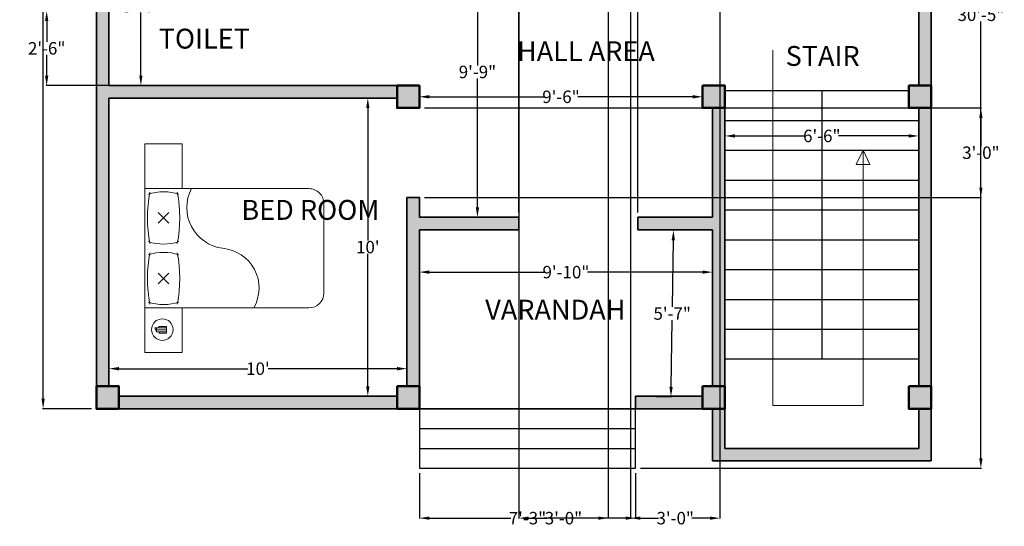
# Model space of a CAD drawing. Units: inches. Extents: x 157 to 553, y 100 to 520.
# Tile 1 of 2: x 157 to 553, y 100 to 304. Entities that reach past the tile are written whole.
import ezdxf

# ---------------------------------------------------------------- set-up
doc = ezdxf.new("R2010")
doc.units = ezdxf.units.IN
doc.header["$MEASUREMENT"] = 0
doc.layers.get('0').update_dxf_attribs({"color": 255})
for name, color, linetype, lineweight in [('A-ANNO-DIMS', 2, 'Continuous', 18), ('A-ANNO-SYMB', 2, 'Continuous', 18), ('A-AREA-IDEN', 7, 'Continuous', 25), ('A-COLS', 7, 'Continuous', 50), ('A-FLOR-STRS', 7, 'Continuous', 25), ('A-FURN', 3, 'Continuous', 18), ('A-WALL', 7, 'Continuous', 35), ('A-WALL-PATT', 3, 'Continuous', 13)]:
    doc.layers.add(name, color=color, linetype=linetype, lineweight=lineweight)
doc.layers.add('A-COLS-PATT', color=18, linetype='Continuous', lineweight=13, true_color=0x000000)
doc.styles.get("Standard").update_dxf_attribs({"font": 'arial.ttf'})
doc.dimstyles.get("Standard").update_dxf_attribs({"dimtxt": 5, "dimasz": 4, "dimexe": 0.18, "dimexo": 2, "dimgap": 0.09, "dimtad": 0, "dimtih": 1, "dimtoh": 1, "dimdec": 0, "dimzin": 0, "dimdsep": 46, "dimlunit": 3, "dimtxsty": 'Standard', "dimcen": 2, "dimadec": 0, "dimazin": 0, "dimtfac": 1, "dimtdec": 0, "dimtofl": 0, "dimtmove": 0, "dimatfit": 3, "dimfxl": 1, "dimtolj": 1, "dimtzin": 0, "dimarcsym": 0})

# ---------------------------------------------------------------- blocks, each defined once
blk = doc.blocks.new('*D2')
at = {"layer": 'A-ANNO-DIMS', "color": 0, "lineweight": -2, "transparency": 16777216}
for p, q in [((185.79, 488.7), (166.12, 488.7)), ((166.3, 484.7), (166.3, 320.85)), ((166.3, 151.7), (166.3, 315.56)), ((185.79, 147.7), (166.12, 147.7))]:
    blk.add_line(p, q, dxfattribs=at)
at = {"layer": 'A-ANNO-DIMS', "color": 0, "transparency": 16777216}
for points in [[(165.64, 484.7), (166.97, 484.7), (166.3, 488.7)], [(165.64, 151.7), (166.97, 151.7), (166.3, 147.7)]]:
    blk.add_solid(points, dxfattribs=at)
at = {"layer": 'Defpoints', "color": 0, "transparency": 16777216}
for p in [(187.79, 488.7), (166.3, 147.7), (187.79, 147.7)]:
    blk.add_point(p, dxfattribs=at)
at = {"layer": 'A-ANNO-DIMS', "color": 0, "transparency": 16777216, "insert": (166.3, 318.2), "char_height": 5, "attachment_point": 5}
blk.add_mtext('\\A1;28\'-5"', dxfattribs=at)
blk = doc.blocks.new('*D3')
at = {"layer": 'A-ANNO-DIMS', "color": 0, "lineweight": -2, "transparency": 16777216}
for p, q in [((440.79, 266.7), (440.79, 257.27)), ((518.79, 266.7), (518.79, 257.27)), ((444.79, 257.45), (473.04, 257.45)), ((514.79, 257.45), (486.54, 257.45))]:
    blk.add_line(p, q, dxfattribs=at)
at = {"layer": 'A-ANNO-DIMS', "color": 0, "transparency": 16777216}
for points in [[(444.79, 258.12), (444.79, 256.78), (440.79, 257.45)], [(514.79, 258.12), (514.79, 256.78), (518.79, 257.45)]]:
    blk.add_solid(points, dxfattribs=at)
at = {"layer": 'Defpoints', "color": 0, "transparency": 16777216}
for p in [(440.79, 268.7), (518.79, 268.7), (518.79, 257.45)]:
    blk.add_point(p, dxfattribs=at)
at = {"layer": 'A-ANNO-DIMS', "color": 0, "transparency": 16777216, "insert": (479.79, 257.45), "char_height": 5, "attachment_point": 5}
blk.add_mtext('\\A1;6\'-6"', dxfattribs=at)
blk = doc.blocks.new('*D13')
at = {"layer": 'A-ANNO-DIMS', "color": 0, "lineweight": -2, "transparency": 16777216}
for p, q in [((198.79, 341.7), (205.83, 341.7)), ((205.65, 337.7), (205.65, 312.34)), ((205.65, 281.7), (205.65, 307.07)), ((198.79, 277.7), (205.83, 277.7))]:
    blk.add_line(p, q, dxfattribs=at)
at = {"layer": 'A-ANNO-DIMS', "color": 0, "transparency": 16777216}
for points in [[(204.99, 337.7), (206.32, 337.7), (205.65, 341.7)], [(204.99, 281.7), (206.32, 281.7), (205.65, 277.7)]]:
    blk.add_solid(points, dxfattribs=at)
at = {"layer": 'Defpoints', "color": 0, "transparency": 16777216}
for p in [(196.79, 341.7), (196.79, 277.7), (205.65, 277.7)]:
    blk.add_point(p, dxfattribs=at)
at = {"layer": 'A-ANNO-DIMS', "color": 0, "transparency": 16777216, "insert": (205.65, 309.7), "char_height": 5, "attachment_point": 5}
blk.add_mtext('\\A1;5\'-4"', dxfattribs=at)
blk = doc.blocks.new('*D14')
at = {"layer": 'A-ANNO-DIMS', "color": 0, "lineweight": -2, "transparency": 16777216}
for p, q in [((192.79, 158.7), (192.79, 163.98)), ((196.79, 163.8), (248.69, 163.8)), ((308.79, 163.8), (256.89, 163.8)), ((312.79, 158.7), (312.79, 163.98))]:
    blk.add_line(p, q, dxfattribs=at)
at = {"layer": 'A-ANNO-DIMS', "color": 0, "transparency": 16777216}
for points in [[(196.79, 164.47), (196.79, 163.13), (192.79, 163.8)], [(308.79, 164.47), (308.79, 163.13), (312.79, 163.8)]]:
    blk.add_solid(points, dxfattribs=at)
at = {"layer": 'Defpoints', "color": 0, "transparency": 16777216}
for p in [(312.79, 163.8), (192.79, 156.7), (312.79, 156.7)]:
    blk.add_point(p, dxfattribs=at)
at = {"layer": 'A-ANNO-DIMS', "color": 0, "transparency": 16777216, "insert": (252.79, 163.8), "char_height": 5, "attachment_point": 5}
blk.add_mtext("\\A1;10'", dxfattribs=at)
blk = doc.blocks.new('*D15')
at = {"layer": 'A-ANNO-DIMS', "color": 0, "lineweight": -2, "transparency": 16777216}
for p, q in [((306.79, 272.7), (296.84, 272.7)), ((297.02, 268.7), (297.02, 215.35)), ((297.02, 156.7), (297.02, 210.06)), ((306.79, 152.7), (296.84, 152.7))]:
    blk.add_line(p, q, dxfattribs=at)
at = {"layer": 'A-ANNO-DIMS', "color": 0, "transparency": 16777216}
for points in [[(296.36, 268.7), (297.69, 268.7), (297.02, 272.7)], [(296.36, 156.7), (297.69, 156.7), (297.02, 152.7)]]:
    blk.add_solid(points, dxfattribs=at)
at = {"layer": 'Defpoints', "color": 0, "transparency": 16777216}
for p in [(297.02, 272.7), (308.79, 272.7), (308.79, 152.7)]:
    blk.add_point(p, dxfattribs=at)
at = {"layer": 'A-ANNO-DIMS', "color": 0, "transparency": 16777216, "insert": (297.02, 212.7), "char_height": 5, "attachment_point": 5}
blk.add_mtext("\\A1;10'", dxfattribs=at)
blk = doc.blocks.new('*D16')
at = {"layer": 'A-ANNO-DIMS', "color": 0, "lineweight": -2, "transparency": 16777216}
for p, q in [((317.79, 217.7), (317.79, 202.47)), ((435.79, 217.7), (435.79, 202.47)), ((321.79, 202.65), (368.11, 202.65)), ((431.79, 202.65), (385.47, 202.65))]:
    blk.add_line(p, q, dxfattribs=at)
at = {"layer": 'A-ANNO-DIMS', "color": 0, "transparency": 16777216}
for points in [[(321.79, 203.32), (321.79, 201.99), (317.79, 202.65)], [(431.79, 203.32), (431.79, 201.99), (435.79, 202.65)]]:
    blk.add_solid(points, dxfattribs=at)
at = {"layer": 'Defpoints', "color": 0, "transparency": 16777216}
for p in [(317.79, 219.7), (435.79, 219.7), (435.79, 202.65)]:
    blk.add_point(p, dxfattribs=at)
at = {"layer": 'A-ANNO-DIMS', "color": 0, "transparency": 16777216, "insert": (376.79, 202.65), "char_height": 5, "attachment_point": 5}
blk.add_mtext('\\A1;9\'-10"', dxfattribs=at)
blk = doc.blocks.new('*D17')
at = {"layer": 'A-ANNO-DIMS', "color": 0, "lineweight": -2, "transparency": 16777216}
for p, q in [((407.79, 219.67), (420.24, 219.49)), ((420, 215.49), (419.6, 188.62)), ((419.12, 156.49), (419.52, 183.36)), ((406.79, 152.67), (419.24, 152.49))]:
    blk.add_line(p, q, dxfattribs=at)
at = {"layer": 'A-ANNO-DIMS', "color": 0, "transparency": 16777216}
for points in [[(419.33, 215.5), (420.67, 215.48), (420.06, 219.49)], [(418.45, 156.5), (419.79, 156.48), (419.06, 152.49)]]:
    blk.add_solid(points, dxfattribs=at)
at = {"layer": 'Defpoints', "color": 0, "transparency": 16777216}
for p in [(405.79, 219.7), (420.06, 219.49), (404.79, 152.7)]:
    blk.add_point(p, dxfattribs=at)
at = {"layer": 'A-ANNO-DIMS', "color": 0, "transparency": 16777216, "insert": (419.56, 185.99), "char_height": 5, "attachment_point": 5}
blk.add_mtext('\\A1;5\'-7"', dxfattribs=at)
blk = doc.blocks.new('*D18')
at = {"layer": 'A-ANNO-DIMS', "color": 0, "lineweight": -2, "transparency": 16777216}
for p, q in [((355.79, 341.7), (340.98, 341.7)), ((341.16, 337.7), (341.16, 285.85)), ((341.16, 228.7), (341.16, 280.56)), ((355.79, 224.7), (340.98, 224.7))]:
    blk.add_line(p, q, dxfattribs=at)
at = {"layer": 'A-ANNO-DIMS', "color": 0, "transparency": 16777216}
for points in [[(340.49, 337.7), (341.82, 337.7), (341.16, 341.7)], [(340.49, 228.7), (341.82, 228.7), (341.16, 224.7)]]:
    blk.add_solid(points, dxfattribs=at)
at = {"layer": 'Defpoints', "color": 0, "transparency": 16777216}
for p in [(341.16, 341.7), (357.79, 341.7), (357.79, 224.7)]:
    blk.add_point(p, dxfattribs=at)
at = {"layer": 'A-ANNO-DIMS', "color": 0, "transparency": 16777216, "insert": (341.16, 283.2), "char_height": 5, "attachment_point": 5}
blk.add_mtext('\\A1;9\'-9"', dxfattribs=at)
blk = doc.blocks.new('*D19')
at = {"layer": 'A-ANNO-DIMS', "color": 0, "lineweight": -2, "transparency": 16777216}
for p, q in [((317.79, 270.7), (317.79, 273.38)), ((321.79, 273.2), (368.05, 273.2)), ((427.79, 273.2), (381.52, 273.2)), ((431.79, 270.7), (431.79, 273.38))]:
    blk.add_line(p, q, dxfattribs=at)
at = {"layer": 'A-ANNO-DIMS', "color": 0, "transparency": 16777216}
for points in [[(321.79, 273.87), (321.79, 272.54), (317.79, 273.2)], [(427.79, 273.87), (427.79, 272.54), (431.79, 273.2)]]:
    blk.add_solid(points, dxfattribs=at)
at = {"layer": 'Defpoints', "color": 0, "transparency": 16777216}
for p in [(431.79, 273.2), (317.79, 268.7), (431.79, 268.7)]:
    blk.add_point(p, dxfattribs=at)
at = {"layer": 'A-ANNO-DIMS', "color": 0, "transparency": 16777216, "insert": (374.79, 273.2), "char_height": 5, "attachment_point": 5}
blk.add_mtext('\\A1;9\'-6"', dxfattribs=at)
blk = doc.blocks.new('BED-DOUBLE-WITH-NIGHTSTANDS')
for p, q in [((0, 72), (18, 72)), ((0, 57), (0, 72)), ((6, 72), (84, 72)), ((18, 72), (18, 6)), ((66, 6), (66, 72)), ((84, 72), (84, 57)), ((9.95, 67.98), (8.32, 67.38)), ((9.95, 67.38), (9.95, 67.98)), ((9.14, 67.38), (9.14, 63.35)), ((32, 66.63), (27.75, 62.4)), ((27.76, 66.64), (31.99, 62.39)), ((56.35, 66.63), (52.1, 62.4)), ((52.11, 66.64), (56.34, 62.39)), ((18, 57), (0, 57)), ((84, 57), (66, 57)), ((24, 0), (60, 0))]:
    blk.add_line(p, q)
for points in [[(8.32, 63.35), (7.8, 63.35), (7.8, 66.31), (8.32, 66.31)], [(8.32, 63.35), (9.95, 63.35), (9.95, 67.38), (8.32, 67.38)], [(9.95, 63.35), (10.59, 63.35), (10.59, 66.42), (9.95, 66.42)]]:
    blk.add_lwpolyline(points, close=True)
blk.add_circle((9.27, 65.01), 4.35)
for centre, radius, start, end in [((54.23, 16.39), 56.63, 100.869, 100.8807), ((54.23, 16.39), 56.63, 79.1193, 79.131), ((40, 64.52), 20.63, 162.5077, 197.4923), ((29.88, 16.39), 54.63, 79.1193, 100.8807), ((19.75, 64.52), 20.62, 342.5077, 17.4923), ((64.35, 64.52), 20.63, 162.5077, 197.4923), ((54.23, 16.39), 54.63, 79.1193, 100.8807), ((44.1, 64.52), 20.62, 342.5077, 17.4923), ((29.88, 112.64), 54.63, 259.1193, 280.8807), ((54.23, 112.64), 54.63, 259.1193, 280.8807), ((58.39, 38.66), 16.52, 62.5747, 172.7011), ((25.97, 42.18), 16.1, 240.3431, 354.9328), ((24, 6), 6, 180, 270), ((60, 6), 6, 270, 0)]:
    blk.add_arc(centre, radius, start, end)
blk = doc.blocks.new('*D23')
at = {"layer": 'A-ANNO-DIMS', "color": 0, "lineweight": -2, "transparency": 16777216}
for p, q in [((525.79, 488.7), (544.02, 488.7)), ((543.84, 484.7), (543.84, 308.85)), ((543.84, 127.7), (543.84, 303.56)), ((406.79, 123.7), (544.02, 123.7))]:
    blk.add_line(p, q, dxfattribs=at)
at = {"layer": 'A-ANNO-DIMS', "color": 0, "transparency": 16777216}
for points in [[(543.17, 484.7), (544.5, 484.7), (543.84, 488.7)], [(543.17, 127.7), (544.5, 127.7), (543.84, 123.7)]]:
    blk.add_solid(points, dxfattribs=at)
at = {"layer": 'Defpoints', "color": 0, "transparency": 16777216}
for p in [(523.79, 488.7), (404.79, 123.7), (543.84, 123.7)]:
    blk.add_point(p, dxfattribs=at)
at = {"layer": 'A-ANNO-DIMS', "color": 0, "transparency": 16777216, "insert": (543.84, 306.2), "char_height": 5, "attachment_point": 5}
blk.add_mtext('\\A1;30\'-5"', dxfattribs=at)
blk = doc.blocks.new('*D25')
at = {"layer": 'A-ANNO-DIMS', "color": 0, "lineweight": -2, "transparency": 16777216}
for p, q in [((357.79, 339.7), (357.79, 103.47)), ((393.79, 339.7), (393.79, 103.47)), ((361.79, 103.65), (369.05, 103.65)), ((389.79, 103.65), (382.52, 103.65))]:
    blk.add_line(p, q, dxfattribs=at)
at = {"layer": 'A-ANNO-DIMS', "color": 0, "transparency": 16777216}
for points in [[(361.79, 104.32), (361.79, 102.99), (357.79, 103.65)], [(389.79, 104.32), (389.79, 102.99), (393.79, 103.65)]]:
    blk.add_solid(points, dxfattribs=at)
at = {"layer": 'Defpoints', "color": 0, "transparency": 16777216}
for p in [(357.79, 341.7), (393.79, 341.7), (393.79, 103.65)]:
    blk.add_point(p, dxfattribs=at)
at = {"layer": 'A-ANNO-DIMS', "color": 0, "transparency": 16777216, "insert": (375.79, 103.65), "char_height": 5, "attachment_point": 5}
blk.add_mtext('\\A1;3\'-0"', dxfattribs=at)
blk = doc.blocks.new('*D26')
at = {"layer": 'A-ANNO-DIMS', "color": 0, "lineweight": -2, "transparency": 16777216}
for p, q in [((402.79, 339.7), (402.79, 103.47)), ((438.79, 339.7), (438.79, 103.47)), ((406.79, 103.65), (414.05, 103.65)), ((434.79, 103.65), (427.52, 103.65))]:
    blk.add_line(p, q, dxfattribs=at)
at = {"layer": 'A-ANNO-DIMS', "color": 0, "transparency": 16777216}
for points in [[(406.79, 104.32), (406.79, 102.99), (402.79, 103.65)], [(434.79, 104.32), (434.79, 102.99), (438.79, 103.65)]]:
    blk.add_solid(points, dxfattribs=at)
at = {"layer": 'Defpoints', "color": 0, "transparency": 16777216}
for p in [(402.79, 341.7), (438.79, 341.7), (438.79, 103.65)]:
    blk.add_point(p, dxfattribs=at)
at = {"layer": 'A-ANNO-DIMS', "color": 0, "transparency": 16777216, "insert": (420.79, 103.65), "char_height": 5, "attachment_point": 5}
blk.add_mtext('\\A1;3\'-0"', dxfattribs=at)
blk = doc.blocks.new('*D27')
at = {"layer": 'A-ANNO-DIMS', "color": 0, "lineweight": -2, "transparency": 16777216}
for p, q in [((269.79, 307.7), (167.56, 307.7)), ((167.74, 303.7), (167.74, 295.35)), ((167.74, 281.7), (167.74, 290.06)), ((306.79, 277.7), (167.56, 277.7))]:
    blk.add_line(p, q, dxfattribs=at)
at = {"layer": 'A-ANNO-DIMS', "color": 0, "transparency": 16777216}
for points in [[(167.07, 303.7), (168.4, 303.7), (167.74, 307.7)], [(167.07, 281.7), (168.4, 281.7), (167.74, 277.7)]]:
    blk.add_solid(points, dxfattribs=at)
at = {"layer": 'Defpoints', "color": 0, "transparency": 16777216}
for p in [(271.79, 307.7), (167.74, 277.7), (308.79, 277.7)]:
    blk.add_point(p, dxfattribs=at)
at = {"layer": 'A-ANNO-DIMS', "color": 0, "transparency": 16777216, "insert": (167.74, 292.7), "char_height": 5, "attachment_point": 5}
blk.add_mtext('\\A1;2\'-6"', dxfattribs=at)
blk = doc.blocks.new('*D28')
at = {"layer": 'A-ANNO-DIMS', "color": 0, "lineweight": -2, "transparency": 16777216}
for p, q in [((319.79, 268.7), (544.02, 268.7)), ((543.84, 264.7), (543.84, 253.35)), ((543.84, 236.7), (543.84, 248.06)), ((319.79, 232.7), (544.02, 232.7))]:
    blk.add_line(p, q, dxfattribs=at)
at = {"layer": 'A-ANNO-DIMS', "color": 0, "transparency": 16777216}
for points in [[(543.17, 264.7), (544.5, 264.7), (543.84, 268.7)], [(543.17, 236.7), (544.5, 236.7), (543.84, 232.7)]]:
    blk.add_solid(points, dxfattribs=at)
at = {"layer": 'Defpoints', "color": 0, "transparency": 16777216}
for p in [(317.79, 268.7), (317.79, 232.7), (543.84, 232.7)]:
    blk.add_point(p, dxfattribs=at)
at = {"layer": 'A-ANNO-DIMS', "color": 0, "transparency": 16777216, "insert": (543.84, 250.7), "char_height": 5, "attachment_point": 5}
blk.add_mtext('\\A1;3\'-0"', dxfattribs=at)
blk = doc.blocks.new('*D29')
at = {"layer": 'A-ANNO-DIMS', "color": 0, "lineweight": -2, "transparency": 16777216}
for p, q in [((357.79, 226.7), (357.79, 508.93)), ((361.79, 508.75), (374.95, 508.75)), ((401.79, 508.75), (388.62, 508.75)), ((405.79, 226.7), (405.79, 508.93))]:
    blk.add_line(p, q, dxfattribs=at)
at = {"layer": 'A-ANNO-DIMS', "color": 0, "transparency": 16777216}
for points in [[(361.79, 509.42), (361.79, 508.09), (357.79, 508.75)], [(401.79, 509.42), (401.79, 508.09), (405.79, 508.75)]]:
    blk.add_solid(points, dxfattribs=at)
at = {"layer": 'Defpoints', "color": 0, "transparency": 16777216}
for p in [(405.79, 508.75), (357.79, 224.7), (405.79, 224.7)]:
    blk.add_point(p, dxfattribs=at)
at = {"layer": 'A-ANNO-DIMS', "color": 0, "transparency": 16777216, "insert": (381.79, 508.75), "char_height": 5, "attachment_point": 5}
blk.add_mtext('\\A1;4\'-0"', dxfattribs=at)
blk = doc.blocks.new('*D30')
at = {"layer": 'A-ANNO-DIMS', "color": 0, "lineweight": -2, "transparency": 16777216}
for p, q in [((317.79, 121.7), (317.79, 103.47)), ((404.79, 121.7), (404.79, 103.47)), ((321.79, 103.65), (354.57, 103.65)), ((400.79, 103.65), (368, 103.65))]:
    blk.add_line(p, q, dxfattribs=at)
at = {"layer": 'A-ANNO-DIMS', "color": 0, "transparency": 16777216}
for points in [[(321.79, 104.32), (321.79, 102.99), (317.79, 103.65)], [(400.79, 104.32), (400.79, 102.99), (404.79, 103.65)]]:
    blk.add_solid(points, dxfattribs=at)
at = {"layer": 'Defpoints', "color": 0, "transparency": 16777216}
for p in [(317.79, 123.7), (404.79, 123.7), (404.79, 103.65)]:
    blk.add_point(p, dxfattribs=at)
at = {"layer": 'A-ANNO-DIMS', "color": 0, "transparency": 16777216, "insert": (361.29, 103.65), "char_height": 5, "attachment_point": 5}
blk.add_mtext('\\A1;7\'-3"', dxfattribs=at)

msp = doc.modelspace()

# ---------------------------------------------------------------- hatches: boundary and pattern name
at = {"layer": 'A-COLS-PATT'}
h = msp.add_hatch(color=256, dxfattribs=at)
h.dxf.hatch_style = 1
h.paths.add_polyline_path([(196.79, 156.7), (187.79, 156.7), (187.79, 147.7), (196.79, 147.7)])
h.paths.add_polyline_path([(317.79, 156.7), (308.79, 156.7), (308.79, 147.7), (317.79, 147.7)])
h.paths.add_polyline_path([(440.79, 156.7), (431.79, 156.7), (431.79, 147.7), (440.79, 147.7)])
h.paths.add_polyline_path([(523.79, 156.7), (514.79, 156.7), (514.79, 147.7), (523.79, 147.7)])
h.paths.add_polyline_path([(523.79, 277.7), (514.79, 277.7), (514.79, 268.7), (523.79, 268.7)])
h.paths.add_polyline_path([(440.79, 277.7), (431.79, 277.7), (431.79, 268.7), (440.79, 268.7)])
h.paths.add_polyline_path([(317.79, 277.7), (308.79, 277.7), (308.79, 268.7), (317.79, 268.7)])
h.paths.add_polyline_path([(196.79, 350.7), (187.79, 350.7), (187.79, 341.7), (196.79, 341.7)])
h.paths.add_polyline_path([(317.79, 350.7), (308.79, 350.7), (308.79, 341.7), (317.79, 341.7)])
h.paths.add_polyline_path([(402.79, 350.7), (393.79, 350.7), (393.79, 341.7), (402.79, 341.7)])
h.paths.add_polyline_path([(523.79, 350.7), (514.79, 350.7), (514.79, 341.7), (523.79, 341.7)])
h.paths.add_polyline_path([(523.79, 488.7), (514.79, 488.7), (514.79, 479.7), (523.79, 479.7)])
h.paths.add_polyline_path([(402.79, 488.7), (393.79, 488.7), (393.79, 479.7), (402.79, 479.7)])
h.paths.add_polyline_path([(317.79, 488.7), (308.79, 488.7), (308.79, 479.7), (317.79, 479.7)])
h.paths.add_polyline_path([(196.79, 488.7), (187.79, 488.7), (187.79, 479.7), (196.79, 479.7)])
at = {"layer": 'A-WALL-PATT'}
h = msp.add_hatch(color=256, dxfattribs=at)
h.dxf.hatch_style = 1
h.paths.add_polyline_path([(271.79, 346.7), (196.79, 346.7), (196.79, 341.7), (266.79, 341.7), (266.79, 307.7), (271.79, 307.7)])
h.paths.add_polyline_path([(308.79, 277.7), (192.79, 277.7), (192.79, 341.7), (187.79, 341.7), (187.79, 156.7), (192.79, 156.7), (192.79, 272.7), (308.79, 272.7)])
h.paths.add_polyline_path([(357.79, 224.7), (317.79, 224.7), (317.79, 232.7), (312.79, 232.7), (312.79, 156.7), (317.79, 156.7), (317.79, 219.7), (357.79, 219.7)])
h.paths.add_polyline_path([(308.79, 152.7), (196.79, 152.7), (196.79, 147.7), (308.79, 147.7)])
h.paths.add_polyline_path([(440.79, 268.7), (435.79, 268.7), (435.79, 224.7), (405.79, 224.7), (405.79, 219.7), (435.79, 219.7), (435.79, 156.7), (440.79, 156.7)])
h.paths.add_polyline_path([(523.79, 147.7), (518.79, 147.7), (518.79, 131.7), (440.79, 131.7), (440.79, 147.7), (435.79, 147.7), (435.79, 126.7), (523.79, 126.7)])
h.paths.add_polyline_path([(523.79, 268.7), (518.79, 268.7), (518.79, 156.7), (523.79, 156.7)])
h.paths.add_polyline_path([(523.79, 341.7), (518.79, 341.7), (518.79, 277.7), (523.79, 277.7)])
h.paths.add_polyline_path([(523.79, 479.7), (518.79, 479.7), (518.79, 350.7), (523.79, 350.7)])
h.paths.add_polyline_path([(514.79, 346.7), (438.79, 346.7), (438.79, 341.7), (514.79, 341.7)])
h.paths.add_polyline_path([(317.79, 430.7), (357.79, 430.7), (357.79, 435.7), (317.79, 435.7), (317.79, 479.7), (312.79, 479.7), (312.79, 350.7), (317.79, 350.7)])
h.paths.add_polyline_path([(357.79, 346.7), (317.79, 346.7), (317.79, 341.7), (357.79, 341.7)])
h.paths.add_polyline_path([(398.79, 479.7), (393.79, 479.7), (393.79, 350.7), (398.79, 350.7)])
h.paths.add_polyline_path([(192.79, 479.7), (187.79, 479.7), (187.79, 350.7), (192.79, 350.7)])
h.paths.add_polyline_path([(308.79, 488.7), (196.79, 488.7), (196.79, 483.7), (308.79, 483.7)])
h.paths.add_polyline_path([(393.79, 488.7), (317.79, 488.7), (317.79, 483.7), (393.79, 483.7)])
h.paths.add_polyline_path([(514.79, 488.7), (402.79, 488.7), (402.79, 483.7), (514.79, 483.7)])
h = msp.add_hatch(color=256, dxfattribs=at)
h.dxf.hatch_style = 1
h.paths.add_polyline_path([(431.79, 152.7), (404.79, 152.7), (404.79, 147.7), (431.79, 147.7)])

# ---------------------------------------------------------------- linework, layer by layer
at = {"layer": 'A-ANNO-SYMB'}
for p, q in [((460.13, 291.98), (460.13, 148.93)), ((496.5, 251.7), (493.65, 246.02)), ((496.5, 148.93), (496.5, 251.7)), ((499.18, 245.96), (496.5, 251.7)), ((493.65, 246.02), (499.18, 245.96)), ((460.13, 148.93), (496.5, 148.93))]:
    msp.add_line(p, q, dxfattribs=at)
at = {"layer": 'A-COLS'}
for points in [[(308.79, 277.7), (317.79, 277.7), (317.79, 268.7), (308.79, 268.7)], [(431.79, 277.7), (440.79, 277.7), (440.79, 268.7), (431.79, 268.7)], [(514.79, 277.7), (523.79, 277.7), (523.79, 268.7), (514.79, 268.7)], [(187.79, 156.7), (196.79, 156.7), (196.79, 147.7), (187.79, 147.7)], [(308.79, 156.7), (317.79, 156.7), (317.79, 147.7), (308.79, 147.7)], [(431.79, 156.7), (440.79, 156.7), (440.79, 147.7), (431.79, 147.7)], [(514.79, 156.7), (523.79, 156.7), (523.79, 147.7), (514.79, 147.7)]]:
    msp.add_lwpolyline(points, close=True, dxfattribs=at)
at = {"layer": 'A-FLOR-STRS'}
for p, q in [((440.79, 275.7), (514.79, 275.7)), ((479.79, 275.7), (479.79, 167.7)), ((440.79, 263.7), (518.79, 263.7)), ((440.79, 251.7), (518.79, 251.7)), ((440.79, 239.7), (518.79, 239.7)), ((440.79, 227.7), (518.79, 227.7)), ((440.79, 215.7), (518.79, 215.7)), ((440.79, 203.7), (518.79, 203.7)), ((440.79, 191.7), (518.79, 191.7)), ((440.79, 179.7), (518.79, 179.7)), ((440.79, 167.7), (518.79, 167.7)), ((317.79, 147.7), (317.79, 123.7)), ((404.79, 123.7), (404.79, 147.7)), ((317.79, 139.7), (404.79, 139.7)), ((317.79, 131.7), (404.79, 131.7)), ((317.79, 123.7), (404.79, 123.7))]:
    msp.add_line(p, q, dxfattribs=at)
at = {"layer": 'A-WALL'}
for p, q in [((187.79, 147.7), (187.79, 488.7)), ((523.79, 488.7), (523.79, 147.7)), ((192.79, 277.7), (192.79, 341.7)), ((518.79, 277.7), (518.79, 341.7)), ((192.79, 277.7), (266.79, 277.7)), ((192.79, 277.7), (317.79, 277.7)), ((317.79, 268.7), (317.79, 277.7)), ((440.79, 147.7), (440.79, 277.7)), ((514.79, 277.7), (523.79, 277.7)), ((192.79, 272.7), (308.79, 272.7)), ((192.79, 156.7), (192.79, 272.7)), ((435.79, 224.7), (435.79, 268.7)), ((518.79, 156.7), (518.79, 268.7)), ((312.79, 156.7), (312.79, 232.7)), ((312.79, 232.7), (317.79, 232.7)), ((317.79, 224.7), (317.79, 232.7)), ((317.79, 224.7), (357.79, 224.7)), ((357.79, 224.7), (357.79, 219.7)), ((405.79, 224.7), (405.79, 219.7)), ((405.79, 224.7), (435.79, 224.7)), ((317.79, 147.7), (317.79, 219.7)), ((317.79, 219.7), (357.79, 219.7)), ((405.79, 219.7), (435.79, 219.7)), ((435.79, 156.7), (435.79, 219.7)), ((196.79, 152.7), (308.79, 152.7)), ((404.79, 147.7), (404.79, 152.7)), ((404.79, 152.7), (431.79, 152.7)), ((440.79, 147.7), (187.79, 147.7)), ((435.79, 147.7), (435.79, 126.7)), ((440.79, 147.7), (440.79, 131.7)), ((523.79, 147.7), (514.79, 147.7)), ((518.79, 131.7), (518.79, 147.7)), ((523.79, 126.7), (523.79, 147.7)), ((440.79, 131.7), (518.79, 131.7)), ((435.79, 126.7), (523.79, 126.7))]:
    msp.add_line(p, q, dxfattribs=at)

# ---------------------------------------------------------------- block references
at = {"layer": 'A-FURN', "rotation": 90.00000000000021}
msp.add_blockref('BED-DOUBLE-WITH-NIGHTSTANDS', (279.32, 170.24), dxfattribs=at)

# ---------------------------------------------------------------- texts
at = {"layer": 'A-AREA-IDEN', "char_height": 8, "attachment_point": 1}
for s, insert in [('{TOILET}', (212.83, 300.6)), ('{HALL AREA}', (357.07, 295.54)), ('{STAIR}', (465.22, 293.64)), ('{BED ROOM}', (246.12, 231.69)), ('{VARANDAH}', (344.29, 191.54))]:
    msp.add_mtext_dynamic_manual_height_columns(s, width=68.988, gutter_width=1, heights=[0], dxfattribs=dict(at, insert=insert))

# ---------------------------------------------------------------- dimensions: what is measured, and where the dimension line sits
at = {"layer": 'A-ANNO-DIMS'}
for base, p1, p2, override, picture, middle in [((405.79, 508.75), (357.79, 224.7), (405.79, 224.7), {"dimdec": 1, "dimlfac": 1, "dimrnd": 0, "dimzin": 1, "dimdsep": 46, "dimlunit": 4, "dimfrac": 2}, '*D29', (381.79, 508.75)), ((393.79, 103.65), (357.79, 341.7), (393.79, 341.7), {"dimdec": 1, "dimlfac": 1, "dimrnd": 0, "dimzin": 1, "dimdsep": 46, "dimlunit": 4, "dimfrac": 2}, '*D25', (375.79, 103.65)), ((438.79, 103.65), (402.79, 341.7), (438.79, 341.7), {"dimdec": 1, "dimlfac": 1, "dimrnd": 0, "dimzin": 1, "dimdsep": 46, "dimlunit": 4, "dimfrac": 2}, '*D26', (420.79, 103.65)), ((431.79, 273.2), (317.79, 268.7), (431.79, 268.7), {"dimclrd": 0, "dimclre": 0, "dimclrt": 0}, '*D19', (374.79, 273.2)), ((518.79, 257.45), (440.79, 268.7), (518.79, 268.7), {"dimclrd": 0, "dimclre": 0, "dimclrt": 0}, '*D3', (479.79, 257.45)), ((435.79, 202.65), (317.79, 219.7), (435.79, 219.7), {"dimclrd": 0, "dimclre": 0, "dimclrt": 0}, '*D16', (376.79, 202.65)), ((312.79, 163.8), (192.79, 156.7), (312.79, 156.7), {"dimclrd": 0, "dimclre": 0, "dimclrt": 0}, '*D14', (252.79, 163.8)), ((404.79, 103.65), (317.79, 123.7), (404.79, 123.7), {"dimdec": 1, "dimlfac": 1, "dimrnd": 0, "dimzin": 1, "dimdsep": 46, "dimlunit": 4, "dimfrac": 2}, '*D30', (361.29, 103.65))]:
    dim = msp.add_linear_dim(base=base, p1=p1, p2=p2, dimstyle='Standard', override=override, dxfattribs=at)
    dim.commit()
    dim.dimension.update_dxf_attribs({"geometry": picture, "text_midpoint": middle})
for base, p1, p2, override, picture, middle in [((166.3, 147.7), (187.79, 488.7), (187.79, 147.7), {"dimclrd": 0, "dimclre": 0, "dimclrt": 0}, '*D2', (166.3, 318.2)), ((543.84, 123.7), (523.79, 488.7), (404.79, 123.7), {"dimdec": 1, "dimlfac": 1, "dimrnd": 0, "dimzin": 1, "dimdsep": 46, "dimlunit": 4, "dimfrac": 2}, '*D23', (543.84, 306.2)), ((205.65, 277.7), (196.79, 341.7), (196.79, 277.7), {"dimclrd": 0, "dimclre": 0, "dimclrt": 0}, '*D13', (205.65, 309.7)), ((341.16, 341.7), (357.79, 224.7), (357.79, 341.7), {"dimclrd": 0, "dimclre": 0, "dimclrt": 0}, '*D18', (341.16, 283.2)), ((167.74, 277.7), (271.79, 307.7), (308.79, 277.7), {"dimdec": 1, "dimlfac": 1, "dimrnd": 0, "dimzin": 1, "dimdsep": 46, "dimlunit": 4, "dimfrac": 2}, '*D27', (167.74, 292.7)), ((297.02, 272.7), (308.79, 152.7), (308.79, 272.7), {"dimclrd": 0, "dimclre": 0, "dimclrt": 0}, '*D15', (297.02, 212.7)), ((543.84, 232.7), (317.79, 268.7), (317.79, 232.7), {"dimdec": 1, "dimlfac": 1, "dimrnd": 0, "dimzin": 1, "dimdsep": 46, "dimlunit": 4, "dimfrac": 2}, '*D28', (543.84, 250.7))]:
    dim = msp.add_linear_dim(base=base, p1=p1, p2=p2, angle=90, dimstyle='Standard', override=override, dxfattribs=at)
    dim.commit()
    dim.dimension.update_dxf_attribs({"geometry": picture, "text_midpoint": middle})
dim = msp.add_aligned_dim(p1=(404.79, 152.7), p2=(405.79, 219.7), distance=-14.27, dimstyle='Standard', override={"dimclrd": 0, "dimclre": 0, "dimclrt": 0}, dxfattribs=at)
dim.commit()
dim.dimension.update_dxf_attribs({"geometry": '*D17', "text_midpoint": (419.56, 185.99)})

doc.saveas('drawing.dxf')
